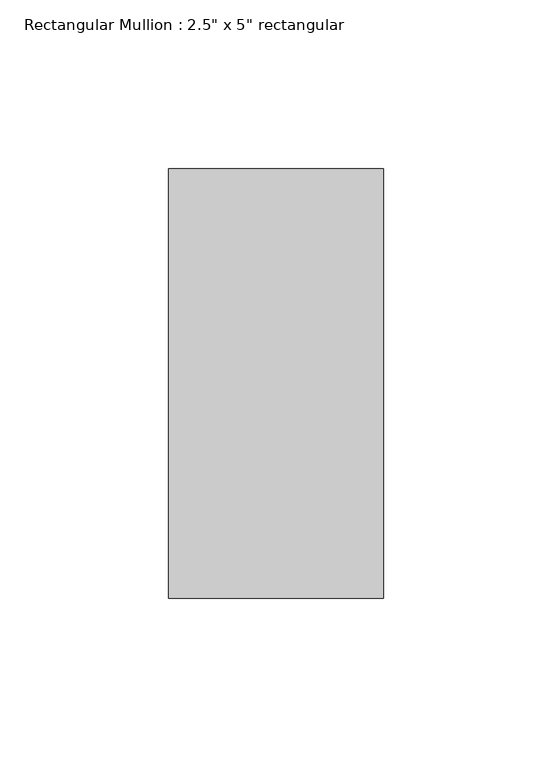
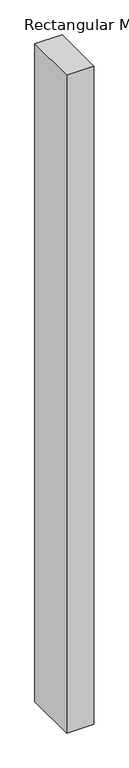
"""IFC4 building model written with IfcOpenShell, lengths in millimetres: member geometry."""

from ifc_helpers import new_model, si_unit, frame, origin, place, context, project, spatial, polyline, outline, extrude, source, transform, mapped, element, save


def member_872f6578(model_context):
    return source(origin(), model_context, "Body", "SweptSolid", [
        extrude(outline(polyline([(31.75, 63.5), (31.75, -63.5), (-31.75, -63.5), (-31.75, 63.5), (31.75, 63.5)])), frame((0.0, 0.0, -1610.0660092), z_axis=(0.0, 0.0, 1.0), x_axis=(1.0, 0.0, 0.0)), (0.0, 0.0, 1.0), 1610.0660092),
    ])


if __name__ == "__main__":
    model = new_model("IFC4")
    model_context = context("Model", 3, world=origin())
    ifc_project = project(units=[si_unit("LENGTHUNIT", "METRE", prefix="MILLI")], contexts=[model_context])
    site = spatial("IfcSite", under=ifc_project)
    building = spatial("IfcBuilding", under=site)
    placement = place(None, origin())
    member_shape = member_872f6578(model_context)
    element("IfcMember", 1, ObjectType="Rectangular Mullion : 2.5\" x 5\" rectangular", at=placement, inside=building, context=model_context, shape_type="MappedRepresentation", body=[
        mapped(member_shape, transform((0.0, 0.0, 0.0), x_axis=(1.0, 0.0, 0.0), y_axis=(0.0, 1.0, 0.0), z_axis=(0.0, 0.0, 1.0))),
    ])
    save(model, "model.ifc")

# Revit data of these elements
# Type "Rectangular Mullion : 2.5\" x 5\" rectangular"
#   built-in parameter 1007304 = 0.416667 (stored number, unit not read)
#   built-in parameter 1007301 = 0.104167 (stored number, unit not read)
#   built-in parameter 1007300 = 0.104167 (stored number, unit not read)
# Element 1 (IfcMember, "Rectangular Mullion : 2.5\" x 5\" rectangular")
#   Materials on its faces: "Aluminum"
# Materials
#   "Aluminum": class "Metal", colour RGB 247 247 247, transparency 0, Description = "Aluminum 6061", Cost = 0
